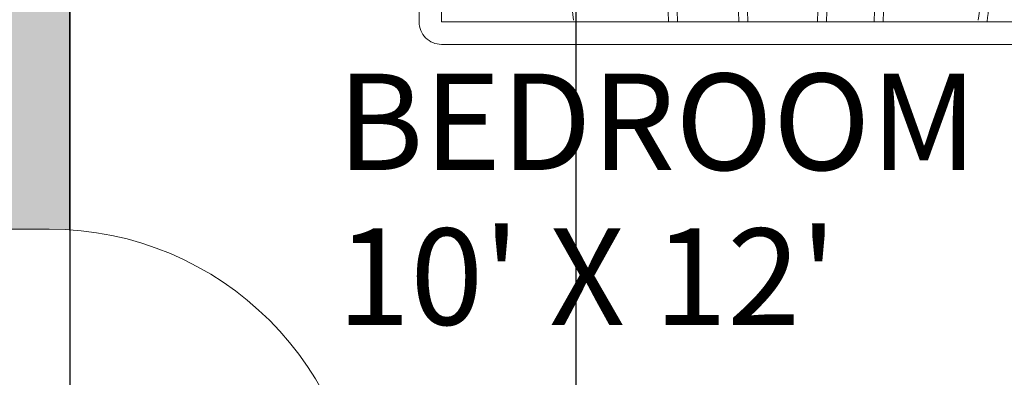
# Model space of a CAD drawing. Units: inches. Extents: x 1763 to 2368, y 1500 to 2097.
# Tile 17 of 24: x 2079 to 2152, y 1856 to 1882. Entities that reach past the tile are written whole.
import ezdxf

# ---------------------------------------------------------------- set-up
doc = ezdxf.new("R2010")
doc.units = ezdxf.units.IN
for name, color, linetype, lineweight in [('A-ANNO-DIMS', 2, 'Continuous', 18), ('A-AREA-IDEN', 7, 'Continuous', 18), ('A-DOOR', 4, 'Continuous', 18), ('A-FURN', 8, 'Continuous', 18), ('A-WALL', 7, 'Continuous', 35), ('A-WALL-PATT', 7, 'Continuous', 13)]:
    doc.layers.add(name, color=color, linetype=linetype, lineweight=lineweight)
doc.styles.get("Standard").update_dxf_attribs({"font": 'arial.ttf'})
doc.dimstyles.new('ISO-25', dxfattribs={"dimtxt": 12.5, "dimasz": 2.5, "dimexe": 1.25, "dimexo": 0.625, "dimtad": 1, "dimdec": 0, "dimlunit": 4, "dimtxsty": 'Standard', "dimblk": 'ARCHTICK', "dimcen": 2.5, "dimclrd": 3, "dimclrt": 4, "dimadec": 0, "dimazin": 0, "dimtfac": 1, "dimtdec": 0, "dimtmove": 0, "dimatfit": 3, "dimfxl": 1, "dimarcsym": 0})

# ---------------------------------------------------------------- blocks, each defined once
blk = doc.blocks.new('A$C77DF40FE')
for p, q in [((2.0097, 2.6214), (2.0097, 0.6344)), ((2.0597, 2.6214), (2.0597, 0.6344)), ((2.0097, 0.6344), (0.5839, 0.6344)), ((2.0097, 0.5844), (0.5839, 0.5844))]:
    blk.add_line(p, q)
for centre, radius, start, end in [((1.3142, -3.5764), 5.4671, 82.7025, 83.4474), ((1.3142, -3.5764), 5.4471, 82.7025, 83.5609), ((1.4138, -15.5462), 17.172, 88.01473, 92.775), ((1.4138, -15.5462), 17.152, 88.01473, 92.775), ((1.4138, -15.6721), 17.172, 88.01473, 92.775), ((1.4138, -15.6721), 17.152, 88.01473, 92.775), ((1.4138, 18.4566), 17.152, 267.225, 271.98527), ((1.4138, 18.4566), 17.172, 267.225, 271.98527), ((1.4138, 18.3004), 17.152, 267.225, 271.98527), ((1.4138, 18.3004), 17.172, 267.225, 271.98527), ((1.3142, 6.3306), 5.4471, 262.3076, 277.2975), ((2.0097, 0.6344), 0.05, 270, 0)]:
    blk.add_arc(centre, radius, start, end)
blk = doc.blocks.new('*U3')
for p, q in [((0, 0), (0, -6)), ((40, 0), (40, -6))]:
    blk.add_line(p, q)
blk.add_lwpolyline([(0, 0), (0, 40), (1.75, 40), (1.75, 0)], close=True)
blk.add_arc((0, 0), 40, 0, 90)
blk = doc.blocks.new('_ArchTick')
at = {"color": 0, "linetype": 'ByBlock', "const_width": 0.15}
blk.add_lwpolyline([(-0.5, -0.5), (0.5, 0.5)], dxfattribs=at)
blk = doc.blocks.new('*D34')
at = {"layer": 'A-ANNO-DIMS', "color": 0, "lineweight": -2, "transparency": 16777216}
for p, q in [((2001.644, 1895.481), (2001.644, 1892.281)), ((2013.092, 1895.481), (2013.092, 1892.281))]:
    blk.add_line(p, q, dxfattribs=at)
at = {"layer": 'A-ANNO-DIMS', "color": 3, "lineweight": -2, "transparency": 16777216}
for p, q in [((2001.644, 1893.531), (2013.092, 1893.531)), ((2013.092, 1893.531), (2131.874, 1893.531))]:
    blk.add_line(p, q, dxfattribs=at)
at = {"layer": 'Defpoints', "color": 0, "transparency": 16777216}
for p in [(2001.644, 1896.106), (2013.092, 1896.106), (2013.092, 1893.531)]:
    blk.add_point(p, dxfattribs=at)
at = {"layer": 'A-ANNO-DIMS', "color": 3, "lineweight": -2, "transparency": 16777216, "xscale": 2.5, "yscale": 2.5, "zscale": 2.5, "rotation": 180}
blk.add_blockref('_ArchTick', (2001.644, 1893.531), dxfattribs=at)
at = {"layer": 'A-ANNO-DIMS', "color": 3, "lineweight": -2, "transparency": 16777216, "xscale": 2.5, "yscale": 2.5, "zscale": 2.5}
blk.add_blockref('_ArchTick', (2013.092, 1893.531), dxfattribs=at)
at = {"layer": 'A-ANNO-DIMS', "color": 4, "transparency": 16777216, "insert": (2073.733, 1900.619), "char_height": 12.5, "attachment_point": 5}
blk.add_mtext('0\'-11 1/2" TYP.', dxfattribs=at)
blk = doc.blocks.new('*D62')
at = {"layer": 'A-ANNO-DIMS', "color": 0, "lineweight": -2, "transparency": 16777216}
for p, q in [((2083.092, 1980.648), (2083.092, 1509.906)), ((2120.612, 1980.648), (2120.612, 1509.906))]:
    blk.add_line(p, q, dxfattribs=at)
at = {"layer": 'A-ANNO-DIMS', "color": 3, "lineweight": -2, "transparency": 16777216}
for p, q in [((2083.092, 1511.156), (2120.612, 1511.156)), ((2120.612, 1511.156), (2186.709, 1511.156))]:
    blk.add_line(p, q, dxfattribs=at)
at = {"layer": 'Defpoints', "color": 0, "transparency": 16777216}
for p in [(2083.092, 1981.273), (2120.612, 1981.273), (2120.612, 1511.156)]:
    blk.add_point(p, dxfattribs=at)
at = {"layer": 'A-ANNO-DIMS', "color": 3, "lineweight": -2, "transparency": 16777216, "xscale": 2.5, "yscale": 2.5, "zscale": 2.5, "rotation": 180}
blk.add_blockref('_ArchTick', (2083.092, 1511.156), dxfattribs=at)
at = {"layer": 'A-ANNO-DIMS', "color": 3, "lineweight": -2, "transparency": 16777216, "xscale": 2.5, "yscale": 2.5, "zscale": 2.5}
blk.add_blockref('_ArchTick', (2120.612, 1511.156), dxfattribs=at)
at = {"layer": 'A-ANNO-DIMS', "color": 4, "transparency": 16777216, "insert": (2154.91, 1518.249), "char_height": 12.5, "attachment_point": 5}
blk.add_mtext('3\'-1 1/2"', dxfattribs=at)
blk = doc.blocks.new('*D71')
at = {"layer": 'A-ANNO-DIMS', "color": 0, "lineweight": -2, "transparency": 16777216}
for p, q in [((2049.686, 1879.648), (2049.686, 1509.906)), ((2072.785, 1879.648), (2072.785, 1509.906))]:
    blk.add_line(p, q, dxfattribs=at)
at = {"layer": 'A-ANNO-DIMS', "color": 3, "lineweight": -2, "transparency": 16777216}
for p, q in [((2049.686, 1511.156), (2072.785, 1511.156)), ((2072.785, 1511.156), (2118.298, 1511.156))]:
    blk.add_line(p, q, dxfattribs=at)
at = {"layer": 'Defpoints', "color": 0, "transparency": 16777216}
for p in [(2049.686, 1880.273), (2072.785, 1880.273), (2072.785, 1511.156)]:
    blk.add_point(p, dxfattribs=at)
at = {"layer": 'A-ANNO-DIMS', "color": 3, "lineweight": -2, "transparency": 16777216, "xscale": 2.5, "yscale": 2.5, "zscale": 2.5, "rotation": 180}
blk.add_blockref('_ArchTick', (2049.686, 1511.156), dxfattribs=at)
at = {"layer": 'A-ANNO-DIMS', "color": 3, "lineweight": -2, "transparency": 16777216, "xscale": 2.5, "yscale": 2.5, "zscale": 2.5}
blk.add_blockref('_ArchTick', (2072.785, 1511.156), dxfattribs=at)
at = {"layer": 'A-ANNO-DIMS', "color": 4, "transparency": 16777216, "insert": (2096.791, 1518.057), "char_height": 12.5, "attachment_point": 5}
blk.add_mtext('1\'-11"', dxfattribs=at)

msp = doc.modelspace()

# ---------------------------------------------------------------- hatches: boundary and pattern name
at = {"layer": 'A-WALL-PATT'}
h = msp.add_hatch(color=256, dxfattribs=at)
h.dxf.hatch_style = 1
h.paths.add_polyline_path([(1838.092, 2034.273), (1838.092, 2043.273), (1829.092, 2043.273), (1829.092, 1953.387), (1838.092, 1953.387)])
h.paths.add_polyline_path([(1838.092, 1913.101), (1829.092, 1913.101), (1829.092, 1862.202), (1838.092, 1862.202)])
h.paths.add_polyline_path([(1838.092, 1825.59), (1829.092, 1825.59), (1829.092, 1738.643), (1838.092, 1738.643)])
h.paths.add_polyline_path([(1895.592, 1885.273), (1838.092, 1885.273), (1838.092, 1880.273), (1895.592, 1880.273)])
h.paths.add_polyline_path([(1857.389, 1784.273), (1838.092, 1784.273), (1838.092, 1779.273), (1857.389, 1779.273)])
h.paths.add_polyline_path([(1958.092, 1981.273), (1971.455, 1981.273), (1971.455, 1986.273), (1968.568, 1986.273), (1958.092, 1986.273), (1953.092, 1986.273), (1927.39, 1986.273), (1927.39, 1981.273), (1953.092, 1981.273), (1953.092, 1885.273), (1932.014, 1885.273), (1932.014, 1880.273), (1959.134, 1880.273), (1959.134, 1883.738), (1959.134, 1885.273), (1958.092, 1885.273)])
h.paths.add_polyline_path([(2018.092, 1981.273), (2031.019, 1981.273), (2031.019, 1986.273), (2018.092, 1986.273), (2013.092, 1986.273), (2001.233, 1986.273), (2001.233, 1981.273), (2013.092, 1981.273), (2013.092, 1885.273), (1982.182, 1885.273, -0.016629), (1982.233, 1883.738), (1982.233, 1880.273), (2049.686, 1880.273), (2049.686, 1883.738, -0.016629), (2049.737, 1885.273), (2018.092, 1885.273)])
h.paths.add_polyline_path([(2083.092, 1981.273), (2120.612, 1981.273), (2120.612, 1986.273), (2083.092, 1986.273), (2078.092, 1986.273), (2063.143, 1986.273), (2063.143, 1981.273), (2078.092, 1981.273), (2078.092, 1885.273), (2072.785, 1885.273), (2072.785, 1883.738), (2072.785, 1880.273), (2078.092, 1880.273), (2078.092, 1866.867), (2081.557, 1866.867, -0.016629), (2083.092, 1866.816)])
h.paths.add_polyline_path([(1871.675, 1635.273), (1838.092, 1635.273), (1838.092, 1626.273), (1871.675, 1626.273)], flags=17)
h.paths.add_polyline_path([(2100.577, 1688.273), (2060.092, 1688.273), (2060.092, 1679.273), (2100.577, 1679.273)], flags=17)
h.paths.add_polyline_path([(2180.092, 1688.273), (2148.744, 1688.273), (2148.744, 1679.273), (2180.092, 1679.273)], flags=17)
h.paths.add_polyline_path([(2189.092, 1746.219), (2180.092, 1746.219), (2180.092, 1743.417), (2180.123, 1743.417), (2180.123, 1726.723), (2180.092, 1572.273), (2034.907, 1572.273), (2034.907, 1565.601), (2034.907, 1563.273), (2189.092, 1563.273)])
h.paths.add_polyline_path([(2060.092, 1802.347, -0.016629), (2058.557, 1802.296), (2055.092, 1802.296), (2055.092, 1635.273), (2042.484, 1635.273), (2042.484, 1629.738), (2042.484, 1626.273), (2055.092, 1626.273), (2055.092, 1599.273), (2040.269, 1599.273), (2040.269, 1590.273), (2060.092, 1590.273)])
h.paths.add_polyline_path([(2019.385, 1629.738, -0.060569), (2020.058, 1635.273), (1995.092, 1635.273), (1990.092, 1635.273), (1927.075, 1635.273), (1927.075, 1626.273), (1990.092, 1626.273), (1990.092, 1590.273), (1995.092, 1590.273), (2005.195, 1590.273), (2005.195, 1599.273), (1995.092, 1599.273), (1995.092, 1626.273), (2019.385, 1626.273)])
edge = h.paths.add_edge_path()
edge.add_line((2180.092, 1837.273), (2167.198, 1837.273))
edge.add_spline(control_points=[(2167.198, 1837.273), (2167.191, 1837.271), (2167.183, 1837.271), (2167.176, 1837.273)], knot_values=[168.955493, 168.955493, 168.955493, 168.955493, 169.065871, 169.065871, 169.065871, 169.065871], degree=3, periodic=0)
edge.add_spline(control_points=[(2167.176, 1837.273), (2166.556, 1837.377), (2166.326, 1846.161), (2165.708, 1846.244)], knot_values=[159.864705, 159.864705, 159.864705, 159.864705, 168.955493, 168.955493, 168.955493, 168.955493], degree=3, periodic=0)
edge.add_line((2167.122, 1837.273), (2163.16, 1837.273))
edge.add_spline(control_points=[(2163.16, 1837.273), (2163.158, 1837.273), (2163.156, 1837.273), (2163.155, 1837.273)], knot_values=[150.537172, 150.537172, 150.537172, 150.537172, 150.553797, 150.553797, 150.553797, 150.553797], degree=3, periodic=0)
edge.add_spline(control_points=[(2163.155, 1837.273), (2162.29, 1837.289), (2161.594, 1846.232), (2160.878, 1846.244)], knot_values=[141.293426, 141.293426, 141.293426, 141.293426, 150.537172, 150.537172, 150.537172, 150.537172], degree=3, periodic=0)
edge.add_line((2163.075, 1837.273), (2158.7, 1837.273))
edge.add_spline(control_points=[(2158.7, 1837.273), (2158.698, 1837.273), (2158.697, 1837.273), (2158.696, 1837.273)], knot_values=[132.033544, 132.033544, 132.033544, 132.033544, 132.049151, 132.049151, 132.049151, 132.049151], degree=3, periodic=0)
edge.add_spline(control_points=[(2158.696, 1837.273), (2157.972, 1837.288), (2157.262, 1846.233), (2156.393, 1846.244)], knot_values=[122.786021, 122.786021, 122.786021, 122.786021, 132.033544, 132.033544, 132.033544, 132.033544], degree=3, periodic=0)
edge.add_line((2158.629, 1837.273), (2153.839, 1837.273))
edge.add_spline(control_points=[(2153.839, 1837.273), (2153.831, 1837.271), (2153.823, 1837.271), (2153.816, 1837.273)], knot_values=[113.451585, 113.451585, 113.451585, 113.451585, 113.562103, 113.562103, 113.562103, 113.562103], degree=3, periodic=0)
edge.add_spline(control_points=[(2153.816, 1837.273), (2153.17, 1837.378), (2152.878, 1846.191), (2152.404, 1846.244)], knot_values=[0, 0, 0, 0, 9.081854, 9.081854, 9.081854, 9.081854], degree=3, periodic=0)
edge.add_line((2153.76, 1837.273), (2150.391, 1837.273))
edge.add_spline(control_points=[(2150.391, 1837.273), (2150.381, 1837.272), (2150.371, 1837.272), (2150.361, 1837.273)], knot_values=[95.069382, 95.069382, 95.069382, 95.069382, 95.17519, 95.17519, 95.17519, 95.17519], degree=3, periodic=0)
edge.add_spline(control_points=[(2150.361, 1837.273), (2149.487, 1837.373), (2148.419, 1846.194), (2147.589, 1846.244)], knot_values=[85.824599, 85.824599, 85.824599, 85.824599, 95.069382, 95.069382, 95.069382, 95.069382], degree=3, periodic=0)
edge.add_line((2150.286, 1837.273), (2145.43, 1837.273))
edge.add_spline(control_points=[(2145.43, 1837.273), (2145.426, 1837.273), (2145.423, 1837.273), (2145.419, 1837.273)], knot_values=[76.505559, 76.505559, 76.505559, 76.505559, 76.547811, 76.547811, 76.547811, 76.547811], degree=3, periodic=0)
edge.add_spline(control_points=[(2145.419, 1837.273), (2144.684, 1837.313), (2143.804, 1846.194), (2142.948, 1846.244)], knot_values=[67.23945, 67.23945, 67.23945, 67.23945, 76.505559, 76.505559, 76.505559, 76.505559], degree=3, periodic=0)
edge.add_line((2145.353, 1837.273), (2134.57, 1837.273))
edge.add_spline(control_points=[(2134.57, 1837.273), (2134.567, 1837.272), (2134.563, 1837.272), (2134.56, 1837.273)], knot_values=[39.001463, 39.001463, 39.001463, 39.001463, 39.045107, 39.045107, 39.045107, 39.045107], degree=3, periodic=0)
edge.add_spline(control_points=[(2134.56, 1837.273), (2133.872, 1837.313), (2133.397, 1845.853), (2132.328, 1846.244)], knot_values=[29.79778, 29.79778, 29.79778, 29.79778, 39.001463, 39.001463, 39.001463, 39.001463], degree=3, periodic=0)
edge.add_line((2134.498, 1837.273), (2128.075, 1837.273))
edge.add_spline(control_points=[(2128.075, 1837.273), (2128.026, 1837.26), (2127.978, 1837.26), (2127.931, 1837.273)], knot_values=[19.482067, 19.482067, 19.482067, 19.482067, 19.869396, 19.869396, 19.869396, 19.869396], degree=3, periodic=0)
edge.add_spline(control_points=[(2125.013, 1846.244), (2126.165, 1844.663), (2126.821, 1837.57), (2127.931, 1837.273)], knot_values=[10.389805, 10.389805, 10.389805, 10.389805, 19.482067, 19.482067, 19.482067, 19.482067], degree=3, periodic=0)
edge.add_line((2127.931, 1837.273), (2083.092, 1837.273))
edge.add_line((2083.092, 1837.273), (2083.092, 1843.768))
edge.add_line((2083.092, 1843.768), (2081.557, 1843.768))
edge.add_line((2081.557, 1843.768), (2078.092, 1843.768))
edge.add_line((2078.092, 1843.768), (2078.092, 1837.273))
edge.add_line((2078.092, 1837.273), (2055.092, 1837.273))
edge.add_line((2055.092, 1837.273), (2055.092, 1825.395))
edge.add_line((2055.092, 1825.395), (2058.557, 1825.395))
edge.add_line((2058.557, 1825.395), (2060.092, 1825.395))
edge.add_line((2060.092, 1825.395), (2060.092, 1832.273))
edge.add_line((2060.092, 1832.273), (2122.437, 1832.273))
edge.add_spline(control_points=[(2122.437, 1832.273), (2122.727, 1832.584), (2123.008, 1832.617), (2123.275, 1832.273)], knot_values=[5.972033, 5.972033, 5.972033, 5.972033, 8.057258, 8.057258, 8.057258, 8.057258], degree=3, periodic=0)
edge.add_line((2123.275, 1832.273), (2137.951, 1832.273))
edge.add_spline(control_points=[(2137.951, 1832.273), (2137.961, 1832.274), (2137.971, 1832.274), (2137.98, 1832.273)], knot_values=[53.926862, 53.926862, 53.926862, 53.926862, 54.030075, 54.030075, 54.030075, 54.030075], degree=3, periodic=0)
edge.add_spline(control_points=[(2139.716, 1825.016), (2139.281, 1825.062), (2138.671, 1832.176), (2137.98, 1832.273)], knot_values=[54.030075, 54.030075, 54.030075, 54.030075, 61.445194, 61.445194, 61.445194, 61.445194], degree=3, periodic=0)
edge.add_line((2138.045, 1832.273), (2140.962, 1832.273))
edge.add_spline(control_points=[(2140.962, 1832.273), (2140.971, 1832.274), (2140.98, 1832.274), (2140.988, 1832.273)], knot_values=[68.854182, 68.854182, 68.854182, 68.854182, 68.971237, 68.971237, 68.971237, 68.971237], degree=3, periodic=0)
edge.add_spline(control_points=[(2143.19, 1825.016), (2142.436, 1825.065), (2141.561, 1832.162), (2140.988, 1832.273)], knot_values=[68.971237, 68.971237, 68.971237, 68.971237, 76.444911, 76.444911, 76.444911, 76.444911], degree=3, periodic=0)
edge.add_line((2141.041, 1832.273), (2145.43, 1832.273))
edge.add_spline(control_points=[(2145.43, 1832.273), (2145.439, 1832.274), (2145.448, 1832.274), (2145.458, 1832.273)], knot_values=[84.039047, 84.039047, 84.039047, 84.039047, 84.124041, 84.124041, 84.124041, 84.124041], degree=3, periodic=0)
edge.add_spline(control_points=[(2148.108, 1825.016), (2147.34, 1825.02), (2146.303, 1832.193), (2145.458, 1832.273)], knot_values=[84.124041, 84.124041, 84.124041, 84.124041, 91.773891, 91.773891, 91.773891, 91.773891], degree=3, periodic=0)
edge.add_line((2145.538, 1832.273), (2150.393, 1832.273))
edge.add_spline(control_points=[(2150.393, 1832.273), (2150.419, 1832.277), (2150.445, 1832.277), (2150.472, 1832.273)], knot_values=[99.381577, 99.381577, 99.381577, 99.381577, 99.573457, 99.573457, 99.573457, 99.573457], degree=3, periodic=0)
edge.add_spline(control_points=[(2153.974, 1825.016), (2153.093, 1825.281), (2151.529, 1832.103), (2150.472, 1832.273)], knot_values=[99.573457, 99.573457, 99.573457, 99.573457, 107.218357, 107.218357, 107.218357, 107.218357], degree=3, periodic=0)
edge.add_line((2150.568, 1832.273), (2155.598, 1832.273))
edge.add_spline(control_points=[(2155.598, 1832.273), (2155.605, 1832.273), (2155.611, 1832.273), (2155.618, 1832.273)], knot_values=[114.933058, 114.933058, 114.933058, 114.933058, 115.013624, 115.013624, 115.013624, 115.013624], degree=3, periodic=0)
edge.add_spline(control_points=[(2158.285, 1825.016), (2157.395, 1825.074), (2156.252, 1832.197), (2155.618, 1832.273)], knot_values=[115.013624, 115.013624, 115.013624, 115.013624, 122.616269, 122.616269, 122.616269, 122.616269], degree=3, periodic=0)
edge.add_line((2155.678, 1832.273), (2165.195, 1832.273))
edge.add_spline(control_points=[(2165.195, 1832.273), (2165.198, 1832.273), (2165.201, 1832.273), (2165.204, 1832.273)], knot_values=[145.488477, 145.488477, 145.488477, 145.488477, 145.516379, 145.516379, 145.516379, 145.516379], degree=3, periodic=0)
edge.add_spline(control_points=[(2167.446, 1825.016), (2166.961, 1825.022), (2166.056, 1832.246), (2165.204, 1832.273)], knot_values=[145.516379, 145.516379, 145.516379, 145.516379, 153.105469, 153.105469, 153.105469, 153.105469], degree=3, periodic=0)
edge.add_line((2165.29, 1832.273), (2168.928, 1832.273))
edge.add_spline(control_points=[(2168.928, 1832.273), (2168.982, 1832.293), (2169.038, 1832.293), (2169.096, 1832.273)], knot_values=[160.517439, 160.517439, 160.517439, 160.517439, 160.939723, 160.939723, 160.939723, 160.939723], degree=3, periodic=0)
edge.add_spline(control_points=[(2171.086, 1828.645), (2170.355, 1830.369), (2169.624, 1832.094), (2169.096, 1832.273)], knot_values=[160.939723, 160.939723, 160.939723, 160.939723, 164.738835, 164.738835, 164.738835, 164.738835], degree=3, periodic=0)
edge.add_line((2169.096, 1832.273), (2180.092, 1832.273))
edge.add_line((2180.092, 1832.273), (2180.092, 1837.273))
h.paths.add_polyline_path([(2189.092, 1885.523), (2180.092, 1885.523), (2180.092, 1813.317), (2180.123, 1813.317), (2180.123, 1796.623), (2180.123, 1795.256), (2189.092, 1795.256)])
h.paths.add_polyline_path([(2180.092, 1986.273), (2166.28, 1986.273), (2166.28, 1981.273), (2180.092, 1981.273)])
h.paths.add_polyline_path([(2189.092, 2043.273), (2180.092, 2043.273), (2180.092, 2034.273), (2180.092, 1934.108), (2189.092, 1934.108)])
h.paths.add_polyline_path([(1838.092, 1681.592), (1829.092, 1681.592), (1829.092, 1563.273), (2003.864, 1563.273), (2003.864, 1565.601), (2003.864, 1572.273), (1838.092, 1572.273)])

# ---------------------------------------------------------------- linework, layer by layer
at = {"layer": 'A-WALL'}
msp.add_line((2083.092, 1866.816), (2083.092, 1981.273), dxfattribs=at)

# ---------------------------------------------------------------- block references
at = {"layer": 'A-DOOR', "xscale": -0.5774759422388936, "yscale": 0.5774759422388936, "zscale": 0.5774759422388936, "rotation": 270}
msp.add_blockref('*U3', (2081.557, 1843.768), dxfattribs=at)
at = {"layer": 'A-FURN', "xscale": 33.38694677217886, "yscale": 33.38694677217886, "zscale": 33.38694677217886, "rotation": 270}
msp.add_blockref('A$C77DF40FE', (2089.477, 1949.352), dxfattribs=at)

# ---------------------------------------------------------------- texts
at = {"layer": 'A-AREA-IDEN'}
for s, p in [('BEDROOM', (2102.919, 1871.258)), ("10' X 12'", (2102.919, 1859.765))]:
    msp.add_text(s, height=7.1545, dxfattribs=at).set_placement(p)

# ---------------------------------------------------------------- dimensions: what is measured, and where the dimension line sits
at = {"layer": 'A-ANNO-DIMS'}
for base, p1, p2, picture, middle in [((2120.612, 1511.156), (2083.092, 1981.273), (2120.612, 1981.273), '*D62', (2154.91, 1518.249)), ((2072.785, 1511.156), (2049.686, 1880.273), (2072.785, 1880.273), '*D71', (2096.791, 1518.057))]:
    dim = msp.add_linear_dim(base=base, p1=p1, p2=p2, dimstyle='ISO-25', override={"dimdec": 1, "dimlfac": 1, "dimrnd": 0, "dimzin": 1, "dimdsep": 46, "dimlunit": 4, "dimfrac": 2}, dxfattribs=at)
    dim.commit()
    dim.dimension.update_dxf_attribs({"geometry": picture, "text_midpoint": middle})
dim = msp.add_linear_dim(base=(2013.092, 1893.531), p1=(2001.644, 1896.106), p2=(2013.092, 1896.106), text='<> TYP.', dimstyle='ISO-25', override={"dimdec": 1, "dimlfac": 1, "dimrnd": 0, "dimzin": 1, "dimdsep": 46, "dimlunit": 4, "dimfrac": 2}, dxfattribs=at)
dim.commit()
dim.dimension.update_dxf_attribs({"geometry": '*D34', "text_midpoint": (2073.733, 1900.619)})

doc.saveas('drawing.dxf')
